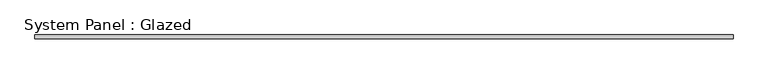
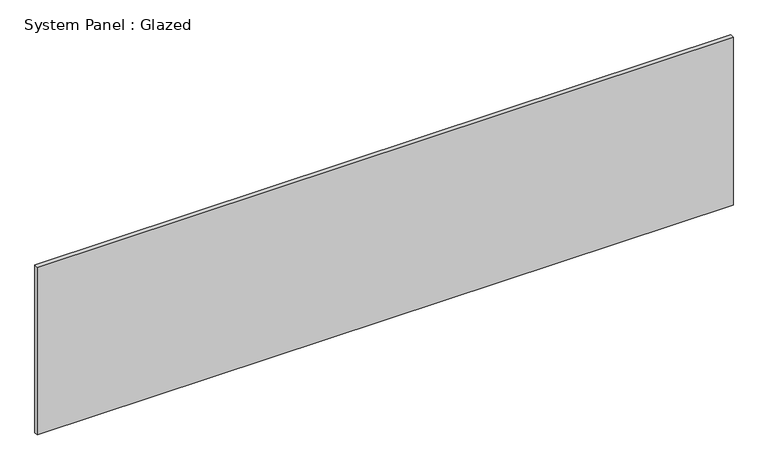
"""IFC4 building model written with IfcOpenShell, lengths in millimetres: plate geometry, System Panel : Glazed."""

from ifc_helpers import new_model, si_unit, origin, origin_with_axes, place, context, project, spatial, polyline, outline, extrude, source, transform, mapped, element, save


def system_panel_glazed_111ae4d9(model_context):
    return source(origin(), model_context, "Body", "SweptSolid", [
        extrude(outline(polyline([(2265.6396657, 19.05), (-2265.6396657, 19.05), (-2265.6396657, 44.45), (2265.6396657, 44.45), (2265.6396657, 19.05)])), origin_with_axes(), (0.0, 0.0, 1.0), 1155.7),
    ])


if __name__ == "__main__":
    model = new_model("IFC4")
    model_context = context("Model", 3, world=origin())
    ifc_project = project(units=[si_unit("LENGTHUNIT", "METRE", prefix="MILLI")], contexts=[model_context])
    site = spatial("IfcSite", under=ifc_project)
    building = spatial("IfcBuilding", under=site)
    placement = place(None, origin())
    system_panel_glazed_shape = system_panel_glazed_111ae4d9(model_context)
    element("IfcPlate", 1, ObjectType="System Panel : Glazed", at=placement, inside=building, context=model_context, shape_type="MappedRepresentation", body=[
        mapped(system_panel_glazed_shape, transform((0.0, 0.0, 0.0), x_axis=(1.0, 0.0, 0.0), y_axis=(0.0, 1.0, 0.0), z_axis=(0.0, 0.0, 1.0))),
    ])
    save(model, "model.ifc")

# Revit data of these elements
# Type "System Panel : Glazed"
#   Construction Type Id = "GSP4R"
#   Analytic Construction = "1/8 in Pilkington single glazing"
#   Visual Light Transmittance = 0.9
#   Solar Heat Gain Coefficient = 0.86
#   Heat Transfer Coefficient (U) = 1.18115 BTU/(h·ft²·°F)
# Element 1 (IfcPlate, "System Panel : Glazed")
#   Materials on its faces: "Glass"
# Materials
#   "Glass": class "Glass", colour RGB 0 128 192, transparency 0.75, Description = "Soda Lime Glass", Cost = 0
